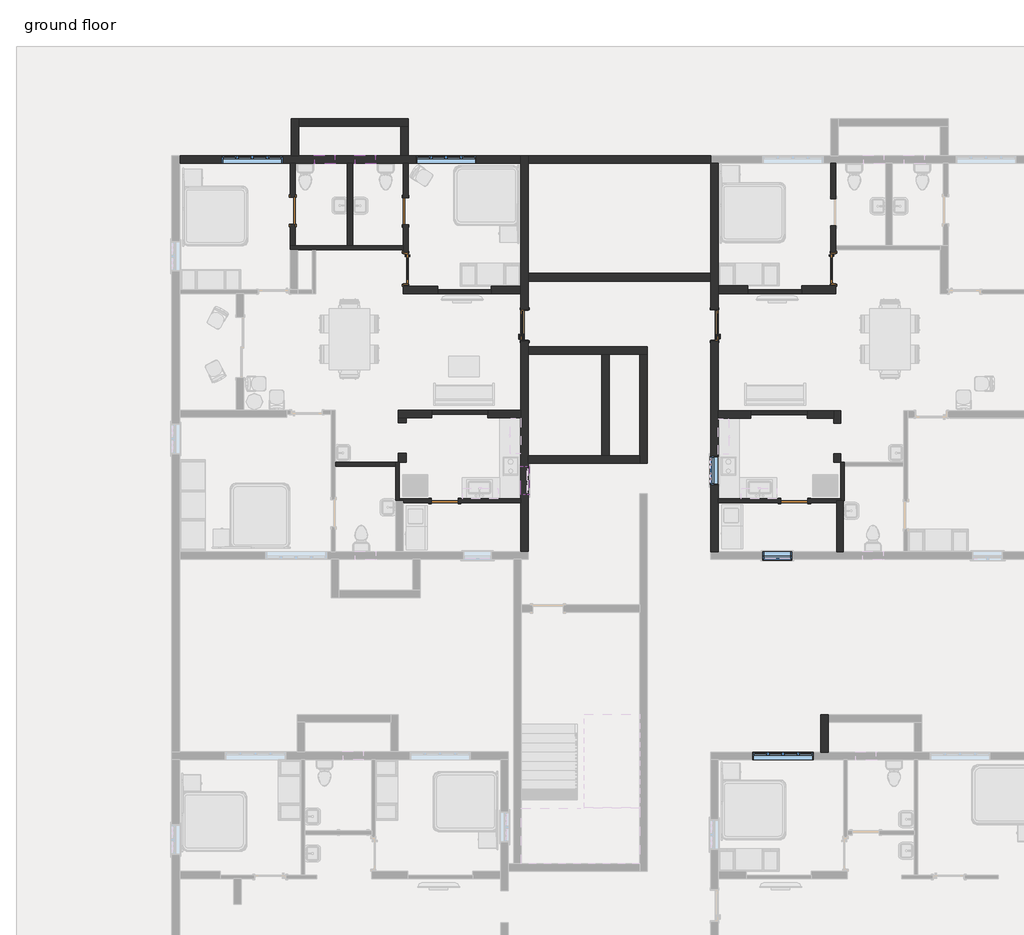
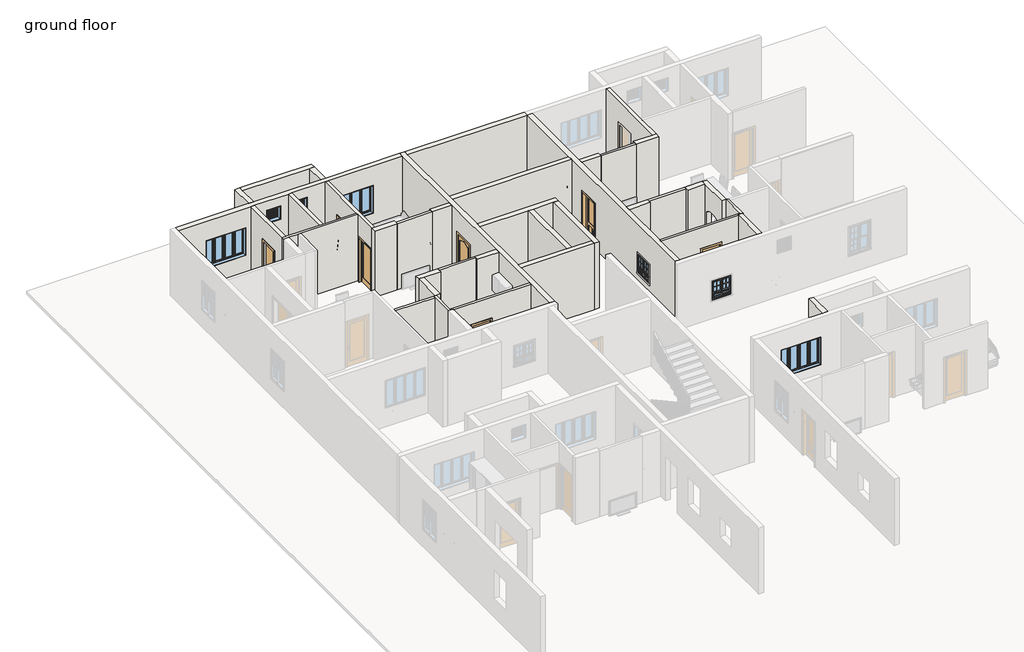
# One storey, part 8 of 16: 38 walls, 8 doors, 8 windows.
# Revit data of these elements (continued)
# Elements 19, 20, 21, 22 (IfcWall, "Generic - 6\"") (continued)
#   Top Offset = 0' - 0"
#   Base Offset = 0' - 0"
#   wall height = 10' - 6"
#   Phase Created = New Construction
#   Base Constraint = ground floor
#   Top Constraint = 1st floor
#   Materials on its faces: "Default Wall"
# Elements 23, 24 (IfcWall, "Generic - 8\"")
#   Top Offset = 0' - 0"
#   Base Offset = 0' - 0"
#   wall height = 10' - 6"
#   Phase Created = New Construction
#   Base Constraint = ground floor
#   Top Constraint = 1st floor
#   Materials on its faces: "Default Wall"
# Elements 25, 26, 27, 28, 29, 30, 31, 32, 33, 34, 35, 36, 37, 38, 39, 40, 41, 42, 43, 44, 45, 46 (IfcWall, "Generic - 9\"")
#   Top Offset = 0' - 0"
#   Base Offset = 0' - 0"
#   wall height = 10' - 6"
#   Phase Created = New Construction
#   Base Constraint = ground floor
#   Top Constraint = 1st floor
#   Materials on its faces: "Default Wall"
# Element 47 (IfcWindow, "Window-Casement-Double-Awning : 34\" x 36\"")
#   Mark = "15"
#   Window Inset = 0' - 0"
#   Interior Wall Closure = 0' - 2 1/4"
#   Frame Extension = 0' - 0 1/4"
#   Exterior Wall Closure = 0' - 1 1/4"
#   Interior Trim Visibility = yes
#   Exterior Trim Visibility = yes
#   Phase Created = New Construction
#   Materials on its faces: "Wood - Stained", "Glass", "Clad - White"
# Element 48 (IfcWindow, "Window-Casement-Double-Awning : 34\" x 36\"")
#   Mark = "70"
#   Window Inset = 0' - 0"
#   Interior Wall Closure = 0' - 2 1/4"
#   Frame Extension = 0' - 0 1/4"
#   Exterior Wall Closure = 0' - 1 1/4"
#   Interior Trim Visibility = yes
#   Exterior Trim Visibility = yes
#   Phase Created = New Construction
#   Materials on its faces: "Wood - Stained", "Glass", "Clad - White"
# Element 49 (IfcWindow, "Window-Casement-Double-Awning : 34\" x 36\"")
#   Mark = "71"
#   Window Inset = 0' - 0"
#   Interior Wall Closure = 0' - 2 1/4"
#   Frame Extension = 0' - 0 1/4"
#   Exterior Wall Closure = 0' - 1 1/4"
#   Interior Trim Visibility = yes
#   Exterior Trim Visibility = yes
#   Phase Created = New Construction
#   Materials on its faces: "Wood - Stained", "Glass", "Clad - White"
# Element 50 (IfcWindow, "Window-Casement-Multi-Sash-Horizontal : 72\" x 53\"")
#   Mark = "11"
#   Window Inset = 0' - 0 5/8"
#   Frame Gap 3 = 0' - 1 83/128"
#   Frame Gap 2 = 0' - 0 5/8"
#   Phase Created = New Construction
#   Materials on its faces: "Metal - Aluminum", "Glass"
# Element 51 (IfcWindow, "Window-Casement-Multi-Sash-Horizontal : 72\" x 53\"")
#   Mark = "12"
#   Window Inset = 0' - 0 5/8"
#   Frame Gap 3 = 0' - 1 83/128"
#   Frame Gap 2 = 0' - 0 5/8"
#   Phase Created = New Construction
#   Materials on its faces: "Metal - Aluminum", "Glass"
# Element 52 (IfcWindow, "Window-Casement-Multi-Sash-Horizontal : 72\" x 53\"")
#   Mark = "20"
#   Window Inset = 0' - 0 5/8"
#   Frame Gap 3 = 0' - 1 83/128"
#   Frame Gap 2 = 0' - 0 5/8"
#   Phase Created = New Construction
#   Materials on its faces: "Metal - Aluminum", "Glass"
# Element 53 (IfcWindow, "Window-Louvers : 24\" x 24\"")
#   Mark = "1"
#   Blade Width = 1' - 10 1/2"
#   Phase Created = New Construction
#   Materials on its faces: "Birch"
# Element 54 (IfcWindow, "Window-Louvers : 24\" x 24\"")
#   Mark = "2"
#   Blade Width = 1' - 10 1/2"
#   Phase Created = New Construction
#   Materials on its faces: "Birch"
# Materials
#   "Cherry": class "Wood", colour RGB 226 177 128, transparency 0, Description = "Prunus Serotina", Cost = 0
#   "Glass": class "Glass", colour RGB 0 128 192, transparency 0.75, Description = "Soda Lime Glass", Cost = 0
#   "Aluminum": class "Metal", colour RGB 247 247 247, transparency 0, Description = "Aluminum 6061", Cost = 0
#   "Door - Panel": class "Wood", colour RGB 210 159 95, transparency 0, Cost = 0
#   "Door - Frame": colour RGB 118 70 51, transparency 0, Cost = 0
#   "Wood - Stained": class "Wood", colour RGB 224 178 126, transparency 0, Cost = 0
#   "Clad - White": class "Wood", colour RGB 242 242 238, transparency 0, Cost = 0
#   "Metal - Aluminum": class "Metal", colour RGB 247 247 247, transparency 0
#   "Birch": class "Wood", colour RGB 224 178 126, transparency 0, Description = "Betula Alleghaniensis", Cost = 0
#   "Default Wall": colour RGB 128 128 128, transparency 0, Cost = 0
